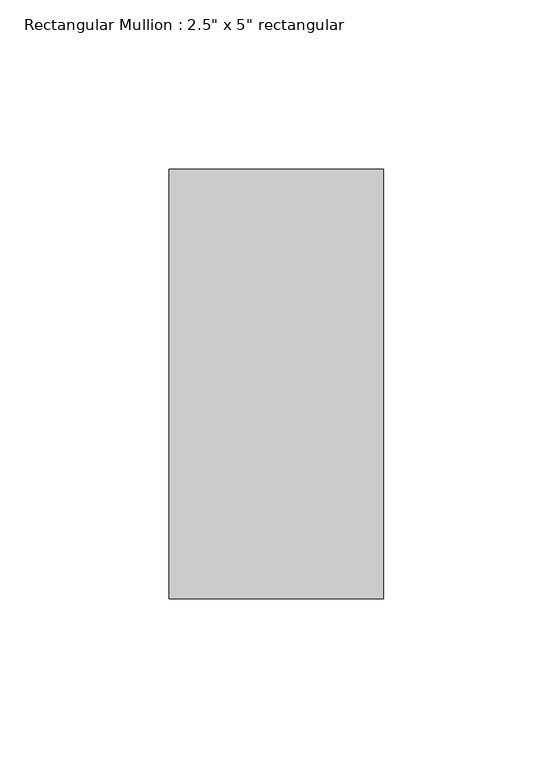
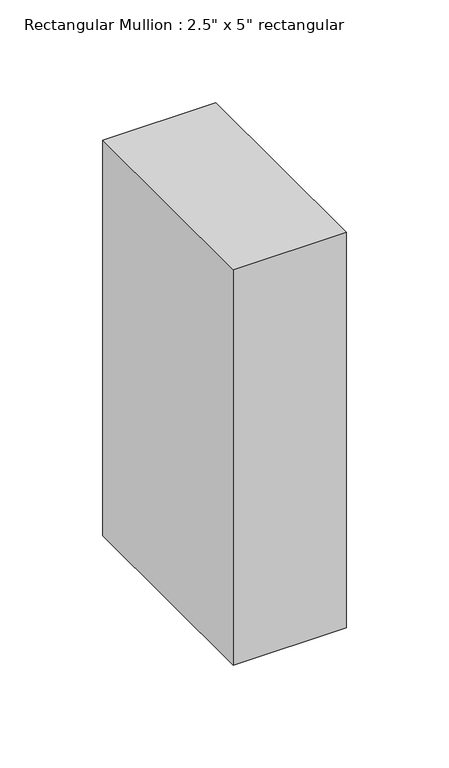
"""IFC4 building model written with IfcOpenShell, lengths in millimetres: member geometry."""

from ifc_helpers import new_model, si_unit, frame, origin, place, context, project, spatial, polyline, outline, extrude, source, transform, mapped, element, save


def member_a608d019(model_context):
    return source(origin(), model_context, "Body", "SweptSolid", [
        extrude(outline(polyline([(0.0, 63.5), (0.0, -63.5), (-63.5, -63.5), (-63.5, 63.5), (0.0, 63.5)])), frame((0.0, 0.0, -234.95), z_axis=(0.0, 0.0, 1.0), x_axis=(1.0, 0.0, 0.0)), (0.0, 0.0, 1.0), 234.95),
    ])


if __name__ == "__main__":
    model = new_model("IFC4")
    model_context = context("Model", 3, world=origin())
    ifc_project = project(units=[si_unit("LENGTHUNIT", "METRE", prefix="MILLI")], contexts=[model_context])
    site = spatial("IfcSite", under=ifc_project)
    building = spatial("IfcBuilding", under=site)
    placement = place(None, origin())
    member_shape = member_a608d019(model_context)
    element("IfcMember", 1, ObjectType="Rectangular Mullion : 2.5\" x 5\" rectangular", at=placement, inside=building, context=model_context, shape_type="MappedRepresentation", body=[
        mapped(member_shape, transform((0.0, 0.0, 0.0), x_axis=(1.0, 0.0, 0.0), y_axis=(0.0, 1.0, 0.0), z_axis=(0.0, 0.0, 1.0))),
    ])
    save(model, "model.ifc")

# Revit data of these elements
# Type "Rectangular Mullion : 2.5\" x 5\" rectangular"
#   built-in parameter 1007304 = 0.416667 (stored number, unit not read)
#   built-in parameter 1007301 = 0.104167 (stored number, unit not read)
#   built-in parameter 1007300 = 0.104167 (stored number, unit not read)
# Element 1 (IfcMember, "Rectangular Mullion : 2.5\" x 5\" rectangular")
#   Materials on its faces: "Aluminum"
# Materials
#   "Aluminum": class "Metal", colour RGB 247 247 247, transparency 0, Description = "Aluminum 6061", Cost = 0
